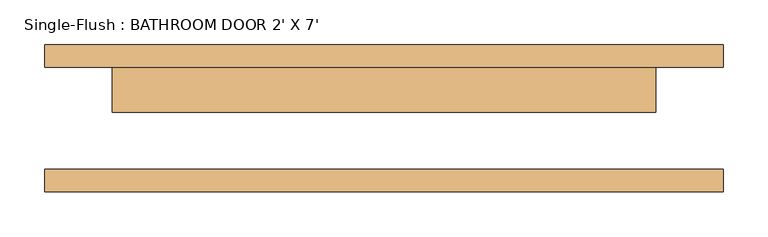
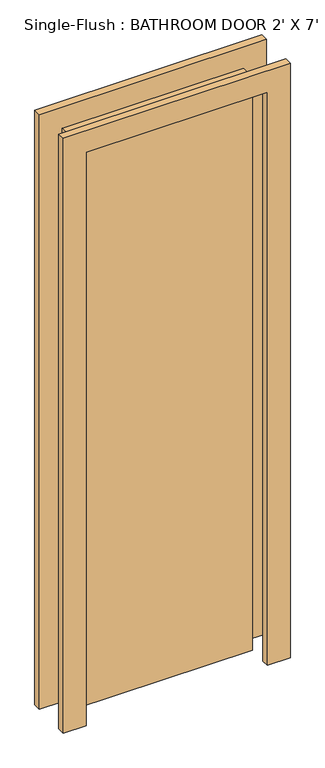
"""IFC4 building model written with IfcOpenShell, lengths in millimetres: door geometry, Single-Flush : BATHROOM DOOR 2' X 7'."""

from ifc_helpers import new_model, si_unit, frame, origin, origin_with_axes, place, context, project, spatial, polyline, outline, extrude, source, transform, mapped, element, save


def single_flush_bathroom_door_2_x_7_d2bb450e(model_context):
    return source(origin(), model_context, "Body", "SweptSolid", [
        extrude(outline(polyline([(2108.2, -381.0), (0.0, -381.0), (0.0, -304.8), (2032.0, -304.8), (2032.0, 304.8), (0.0, 304.8), (0.0, 381.0), (2108.2, 381.0), (2108.2, -381.0)])), frame((0.0, 57.15, 0.0), z_axis=(0.0, 1.0, 0.0), x_axis=(0.0, 0.0, 1.0)), (0.0, 0.0, 1.0), 25.4),
        extrude(outline(polyline([(2108.2, 381.0), (2108.2, -381.0), (0.0, -381.0), (0.0, -304.8), (2032.0, -304.8), (2032.0, 304.8), (0.0, 304.8), (0.0, 381.0), (2108.2, 381.0)])), frame((0.0, -82.55, 0.0), z_axis=(0.0, 1.0, 0.0), x_axis=(0.0, 0.0, 1.0)), (0.0, 0.0, 1.0), 25.4),
        extrude(outline(polyline([(304.8, 6.35), (-304.8, 6.35), (-304.8, 57.15), (304.8, 57.15), (304.8, 6.35)])), origin_with_axes(), (0.0, 0.0, 1.0), 2032.0),
    ])


if __name__ == "__main__":
    model = new_model("IFC4")
    model_context = context("Model", 3, world=origin())
    ifc_project = project(units=[si_unit("LENGTHUNIT", "METRE", prefix="MILLI")], contexts=[model_context])
    site = spatial("IfcSite", under=ifc_project)
    building = spatial("IfcBuilding", under=site)
    placement = place(None, origin())
    single_flush_bathroom_door_2_x_7_shape = single_flush_bathroom_door_2_x_7_d2bb450e(model_context)
    element("IfcDoor", 1, ObjectType="Single-Flush : BATHROOM DOOR 2' X 7'", at=placement, inside=building, context=model_context, shape_type="MappedRepresentation", body=[
        mapped(single_flush_bathroom_door_2_x_7_shape, transform((0.0, 0.0, 0.0), x_axis=(1.0, 0.0, 0.0), y_axis=(0.0, 1.0, 0.0), z_axis=(0.0, 0.0, 1.0))),
    ])
    save(model, "model.ifc")

# Revit data of these elements
# Type "Single-Flush : BATHROOM DOOR 2' X 7'"
#   Type Mark = "11"
#   Construction Type Id = "MDOOR"
#   Assembly Code = "C1020"
#   Analytic Construction = "Metal"
#   Thickness = 0' - 2"
#   Heat Transfer Coefficient (U) = 0.651978 BTU/(h·ft²·°F)
#   Height = 6' - 8"
#   Trim Projection Ext = 0' - 1"
#   Trim Projection Int = 0' - 1"
#   Trim Width = 0' - 3"
#   Width = 2' - 0"
#   Define Thermal Properties by = 1
#   Door Material = Door - Panel
#   Frame Material = Door - Frame
#   Visual Light Transmittance = 0
#   Solar Heat Gain Coefficient = 0
#   Function = (empty or 0)
#   Wall Closure = (empty or 0)
# Element 1 (IfcDoor, "Single-Flush : BATHROOM DOOR 2' X 7'")
#   Materials on its faces: "Door - Frame", "Door - Panel"
# Materials
#   "Door - Panel": class "Wood", colour RGB 210 159 95, transparency 0, Cost = 0
#   "Door - Frame": colour RGB 118 70 51, transparency 0, Cost = 0
